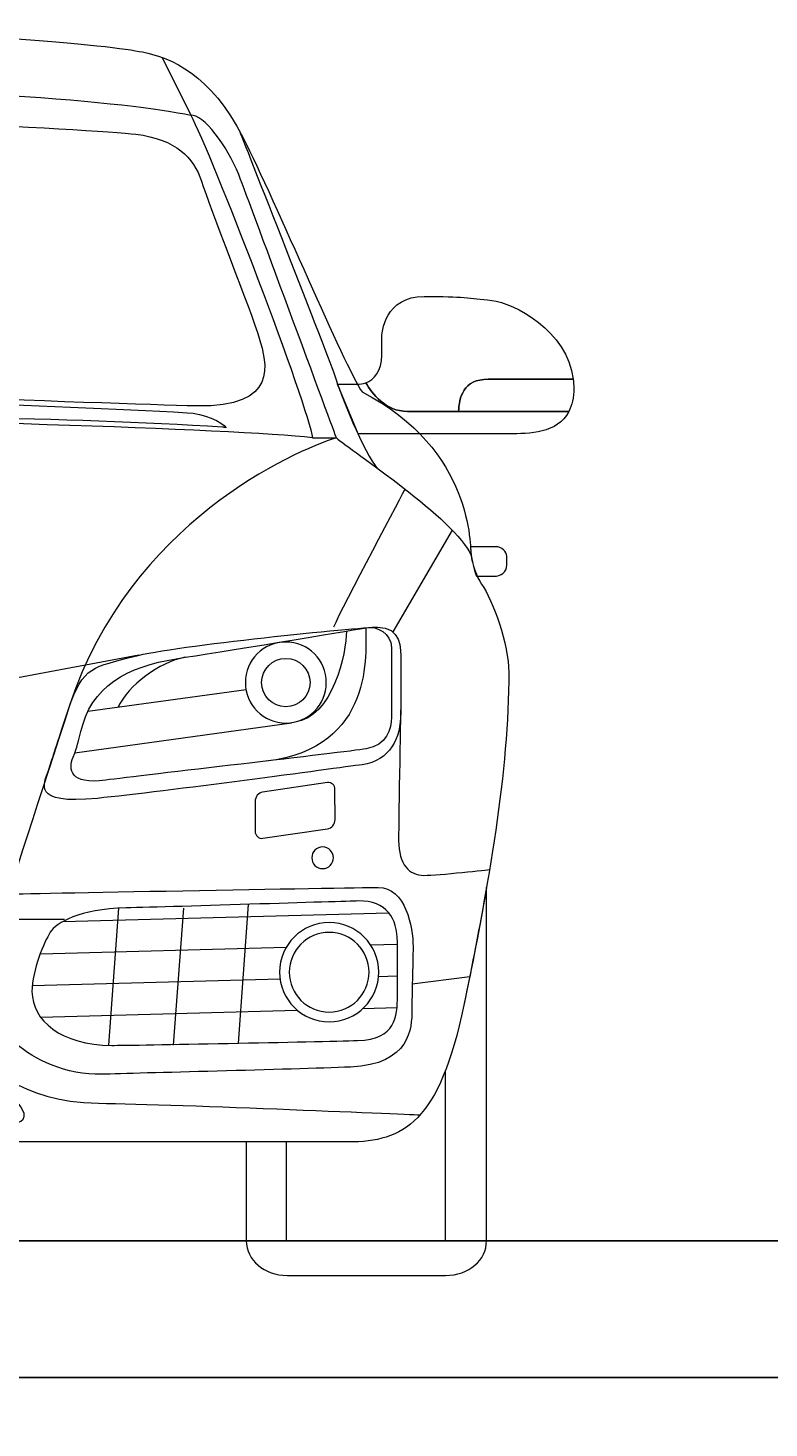
# Model space of a CAD drawing. Units: inches. Extents: x 1152 to 2588, y 1459 to 2618.
# Tile 11 of 17: x 1352 to 1384, y 2319 to 2381. Entities that reach past the tile are written whole.
import ezdxf

# ---------------------------------------------------------------- set-up
doc = ezdxf.new("R2010")
doc.units = ezdxf.units.IN
for name, color, linetype, lineweight in [('A-ANNO-DIMS', 2, 'Continuous', 18), ('A-ELEV', 7, 'Continuous', 25), ('AUDI', 7, 'Continuous', 13)]:
    doc.layers.add(name, color=color, linetype=linetype, lineweight=lineweight)
doc.styles.get("Standard").update_dxf_attribs({"font": 'arial.ttf'})
doc.dimstyles.get("Standard").update_dxf_attribs({"dimtxt": 0.18, "dimasz": 0.18, "dimexe": 0.18, "dimexo": 0.0625, "dimgap": 0.09, "dimtad": 0, "dimtih": 1, "dimtoh": 1, "dimdec": 4, "dimzin": 0, "dimdsep": 46, "dimtxsty": 'Standard', "dimcen": 0.09, "dimadec": 0, "dimazin": 0, "dimtfac": 1, "dimtdec": 4, "dimtofl": 0, "dimtmove": 0, "dimatfit": 3, "dimfxl": 1, "dimtolj": 1, "dimtzin": 0, "dimarcsym": 0})

# ---------------------------------------------------------------- blocks, each defined once
blk = doc.blocks.new('*D91')
at = {"layer": 'A-ANNO-DIMS', "color": 0, "lineweight": -2, "transparency": 16777216}
for p, q in [((1405.417, 2327.329), (1405.417, 2232.94)), ((1276.417, 2321.329), (1276.417, 2232.94)), ((1276.597, 2233.12), (1340.636, 2233.12)), ((1405.237, 2233.12), (1341.197, 2233.12))]:
    blk.add_line(p, q, dxfattribs=at)
at = {"layer": 'A-ANNO-DIMS', "color": 0, "transparency": 16777216}
for points in [[(1276.597, 2233.15), (1276.597, 2233.09), (1276.417, 2233.12)], [(1405.237, 2233.15), (1405.237, 2233.09), (1405.417, 2233.12)]]:
    blk.add_solid(points, dxfattribs=at)
at = {"layer": 'Defpoints', "color": 0, "transparency": 16777216}
for p in [(1405.417, 2327.391), (1276.417, 2321.391), (1405.417, 2233.12)]:
    blk.add_point(p, dxfattribs=at)
at = {"layer": 'A-ANNO-DIMS', "color": 0, "transparency": 16777216, "insert": (1340.917, 2233.12), "char_height": 0.18, "attachment_point": 5}
blk.add_mtext('\\A1;129', dxfattribs=at)

msp = doc.modelspace()

# ---------------------------------------------------------------- linework, layer by layer
at = {"layer": 'A-ELEV'}
for p, q in [((1736.4165, 2327.3911), (1285.4165, 2327.3911)), ((1736.4165, 2321.3911), (1276.4165, 2321.3911))]:
    msp.add_line(p, q, dxfattribs=at)
at = {"layer": 'AUDI'}
for points, knots in [([(1335.9514, 2380.6082), (1323.07, 2380.6082), (1316.2344, 2379.8209), (1314.9649, 2379.5565), (1314.9649, 2379.5565), (1313.6952, 2379.292), (1311.974, 2378.5979), (1310.5458, 2375.7943), (1310.5458, 2375.7943), (1309.1176, 2372.9909), (1306.1088, 2365.771), (1305.3217, 2364.6395), (1305.3217, 2364.6395), (1300.4024, 2362.1057), (1300.5918, 2357.8087), (1300.5428, 2357.4642), (1300.5428, 2357.4642), (1300.4936, 2357.1198), (1300.2995, 2356.5002), (1300.0824, 2356.2017), (1300.0824, 2356.2017), (1299.5785, 2355.5088), (1298.8858, 2353.5262), (1298.8858, 2352.3397), (1298.8858, 2352.3397), (1298.8858, 2347.9967), (1299.7554, 2343.0506), (1300.8566, 2337.73), (1300.8566, 2337.73), (1301.9224, 2332.5811), (1303.5104, 2331.7248), (1305.9177, 2331.7248), (1305.9177, 2331.7248), (1307.7191, 2331.725), (1335.9514, 2331.7248), (1335.9514, 2331.7248), (1335.9514, 2331.7248), (1335.9514, 2331.725), (1364.1837, 2331.7248), (1365.9852, 2331.7248), (1365.9852, 2331.7248), (1368.3925, 2331.725), (1369.9807, 2332.581), (1371.0466, 2337.73), (1371.0466, 2337.73), (1372.1483, 2343.0506), (1373.0181, 2347.9966), (1373.0181, 2352.3397), (1373.0181, 2352.3397), (1373.0181, 2353.5264), (1372.3251, 2355.5087), (1371.8212, 2356.2017), (1371.8212, 2356.2017), (1371.6039, 2356.5003), (1371.41, 2357.1198), (1371.3608, 2357.4642), (1371.3608, 2357.4642), (1371.3116, 2357.8087), (1371.501, 2362.1057), (1366.5811, 2364.6395), (1366.5811, 2364.6395), (1365.7941, 2365.7711), (1362.7853, 2372.9908), (1361.357, 2375.7943), (1361.357, 2375.7943), (1359.9288, 2378.5979), (1358.2076, 2379.292), (1356.9379, 2379.5565), (1356.9379, 2379.5565), (1355.6684, 2379.821), (1348.8329, 2380.608), (1335.9514, 2380.6082)], [0, 0, 0, 0, 0.0555556, 0.0555556, 0.0555556, 0.0555556, 0.1111111, 0.1111111, 0.1111111, 0.1111111, 0.1666667, 0.1666667, 0.1666667, 0.1666667, 0.2222222, 0.2222222, 0.2222222, 0.2222222, 0.2777778, 0.2777778, 0.2777778, 0.2777778, 0.3333333, 0.3333333, 0.3333333, 0.3333333, 0.3888889, 0.3888889, 0.3888889, 0.3888889, 0.4444444, 0.4444444, 0.4444444, 0.4444445, 0.5, 0.5, 0.5, 0.5, 0.5555556, 0.5555556, 0.5555556, 0.5555556, 0.6111111, 0.6111111, 0.6111111, 0.6111111, 0.6666667, 0.6666667, 0.6666667, 0.6666667, 0.7222222, 0.7222222, 0.7222222, 0.7222222, 0.7777778, 0.7777778, 0.7777778, 0.7777778, 0.8333333, 0.8333333, 0.8333333, 0.8333333, 0.8888889, 0.8888889, 0.8888889, 0.8888889, 0.9444444, 0.9444444, 0.9444444, 0.9444445, 1, 1, 1, 1]), ([(1335.9514, 2380.6082), (1323.07, 2380.6082), (1316.2344, 2379.8209), (1314.9649, 2379.5565), (1314.9649, 2379.5565), (1313.6952, 2379.292), (1311.974, 2378.5979), (1310.5458, 2375.7943), (1310.5458, 2375.7943), (1309.1176, 2372.9909), (1306.1088, 2365.771), (1305.3217, 2364.6395), (1305.3217, 2364.6395), (1300.4024, 2362.1057), (1300.5918, 2357.8087), (1300.5428, 2357.4642), (1300.5428, 2357.4642), (1300.4936, 2357.1198), (1300.2995, 2356.5002), (1300.0824, 2356.2017), (1300.0824, 2356.2017), (1299.5785, 2355.5088), (1298.8858, 2353.5262), (1298.8858, 2352.3397), (1298.8858, 2352.3397), (1298.8858, 2347.9967), (1299.7554, 2343.0506), (1300.8566, 2337.73), (1300.8566, 2337.73), (1301.9224, 2332.5811), (1303.5104, 2331.7248), (1305.9177, 2331.7248), (1305.9177, 2331.7248), (1307.7191, 2331.725), (1335.9514, 2331.7248), (1335.9514, 2331.7248), (1335.9514, 2331.7248), (1335.9514, 2331.7248), (1364.1837, 2331.7248), (1365.9852, 2331.7248), (1365.9852, 2331.7248), (1368.3925, 2331.725), (1369.9807, 2332.581), (1371.0466, 2337.73), (1371.0466, 2337.73), (1372.1483, 2343.0506), (1373.0181, 2347.9966), (1373.0181, 2352.3397), (1373.0181, 2352.3397), (1373.0181, 2353.5264), (1372.3251, 2355.5087), (1371.8212, 2356.2017), (1371.8212, 2356.2017), (1371.6039, 2356.5003), (1371.41, 2357.1198), (1371.3608, 2357.4642), (1371.3608, 2357.4642), (1371.3116, 2357.8087), (1371.501, 2362.1057), (1366.5811, 2364.6395), (1366.5811, 2364.6395), (1365.7941, 2365.7711), (1362.7853, 2372.9908), (1361.357, 2375.7943), (1361.357, 2375.7943), (1359.9288, 2378.5979), (1358.2076, 2379.292), (1356.9379, 2379.5565), (1356.9379, 2379.5565), (1355.6684, 2379.821), (1348.8329, 2380.608), (1335.9514, 2380.6082)], [0, 0, 0, 0, 0.0555556, 0.0555556, 0.0555556, 0.0555556, 0.1111111, 0.1111111, 0.1111111, 0.1111111, 0.1666667, 0.1666667, 0.1666667, 0.1666667, 0.2222222, 0.2222222, 0.2222222, 0.2222222, 0.2777778, 0.2777778, 0.2777778, 0.2777778, 0.3333333, 0.3333333, 0.3333333, 0.3333333, 0.3888889, 0.3888889, 0.3888889, 0.3888889, 0.4444444, 0.4444444, 0.4444444, 0.4444445, 0.5, 0.5, 0.5, 0.5, 0.5555556, 0.5555556, 0.5555556, 0.5555556, 0.6111111, 0.6111111, 0.6111111, 0.6111111, 0.6666667, 0.6666667, 0.6666667, 0.6666667, 0.7222222, 0.7222222, 0.7222222, 0.7222222, 0.7777778, 0.7777778, 0.7777778, 0.7777778, 0.8333333, 0.8333333, 0.8333333, 0.8333333, 0.8888889, 0.8888889, 0.8888889, 0.8888889, 0.9444444, 0.9444444, 0.9444444, 0.9444445, 1, 1, 1, 1]), ([(1335.9514, 2378.0831), (1323.862, 2378.0831), (1315.9013, 2377.3042), (1312.8453, 2376.7794), (1312.8453, 2376.7794), (1311.9763, 2375.2275), (1307.631, 2363.8673), (1307.5068, 2362.6256), (1307.5068, 2362.6256), (1310.8591, 2362.9982), (1325.7217, 2363.4947), (1335.9514, 2363.4947), (1335.9514, 2363.4947), (1346.1812, 2363.4947), (1361.0438, 2362.998), (1364.396, 2362.6256), (1364.396, 2362.6256), (1364.2719, 2363.8675), (1359.9266, 2375.2274), (1359.0575, 2376.7794), (1359.0575, 2376.7794), (1356.4376, 2377.3639), (1348.0408, 2378.0829), (1335.9514, 2378.0831)], [0, 0, 0, 0, 0.1666667, 0.1666667, 0.1666667, 0.1666667, 0.3333333, 0.3333333, 0.3333333, 0.3333333, 0.5, 0.5, 0.5, 0.5, 0.6666667, 0.6666667, 0.6666667, 0.6666667, 0.8333333, 0.8333333, 0.8333333, 0.8333333, 1, 1, 1, 1]), ([(1335.9514, 2376.8669), (1331.6617, 2376.8669), (1317.0146, 2376.1677), (1315.2481, 2375.9467), (1315.2481, 2375.9467), (1313.4816, 2375.7259), (1312.7088, 2374.9163), (1312.3775, 2373.8859), (1312.3775, 2373.8859), (1312.0463, 2372.8554), (1310.1695, 2368.1078), (1309.8383, 2367.0037), (1309.8383, 2367.0037), (1309.5071, 2365.8998), (1308.9561, 2363.9401), (1312.5985, 2364.0229), (1312.5985, 2364.0229), (1316.4298, 2364.1101), (1333.6902, 2364.7958), (1335.9514, 2364.7958), (1335.9514, 2364.7958), (1338.2126, 2364.7959), (1355.473, 2364.1101), (1359.3043, 2364.0229), (1359.3043, 2364.0229), (1362.9467, 2363.9401), (1362.3958, 2365.8997), (1362.0646, 2367.0037), (1362.0646, 2367.0037), (1361.7334, 2368.1079), (1359.8565, 2372.8554), (1359.5253, 2373.8859), (1359.5253, 2373.8859), (1359.1941, 2374.9164), (1358.4212, 2375.7259), (1356.6547, 2375.9467), (1356.6547, 2375.9467), (1354.8882, 2376.1677), (1340.2411, 2376.8668), (1335.9514, 2376.8669)], [0, 0, 0, 0, 0.1, 0.1, 0.1, 0.1, 0.2, 0.2, 0.2, 0.2, 0.3, 0.3, 0.3, 0.3, 0.4, 0.4, 0.4, 0.4, 0.5, 0.5, 0.5, 0.5, 0.6, 0.6, 0.6, 0.6, 0.7, 0.7, 0.7, 0.7, 0.8, 0.8, 0.8, 0.8, 0.9, 0.9, 0.9, 0.9, 1, 1, 1, 1]), ([(1364.396, 2362.6256), (1364.2719, 2363.8675), (1359.9266, 2375.2274), (1359.0575, 2376.7794), (1359.0575, 2376.7794), (1359.616, 2376.8414), (1360.6567, 2375.4309), (1361.168, 2374.1721), (1361.168, 2374.1721), (1361.3562, 2373.7086), (1365.4512, 2362.6256), (1365.4512, 2362.6256), (1365.4512, 2362.6256), (1365.4512, 2362.6256), (1364.396, 2362.6256), (1364.396, 2362.6256)], [0, 0, 0, 0, 0.25, 0.25, 0.25, 0.25, 0.5, 0.5, 0.5, 0.5, 0.75, 0.75, 0.75, 0.75, 1, 1, 1, 1]), ([(1361.2043, 2376.0821), (1361.2043, 2376.0821), (1365.2184, 2365.9026), (1365.3948, 2365.3031), (1365.3948, 2365.3031), (1365.5714, 2364.7035), (1366.6742, 2361.8719), (1367.2738, 2361.2722)], [0, 0, 0, 0, 0.5, 0.5, 0.5, 0.5, 1, 1, 1, 1]), ([(1372.1131, 2365.1973), (1373.0816, 2365.1973), (1374.868, 2365.1973), (1375.8424, 2365.1973), (1375.8424, 2365.1973), (1375.5815, 2367.3215), (1373.237, 2368.5533), (1372.2716, 2368.6531), (1372.2716, 2368.6531), (1371.2487, 2368.759), (1371.0374, 2368.8293), (1369.3093, 2368.8293), (1369.3093, 2368.8293), (1367.5813, 2368.8294), (1367.4403, 2367.2778), (1367.4403, 2366.925), (1367.4403, 2366.925), (1367.4403, 2366.5723), (1367.4403, 2366.7135), (1367.4403, 2366.2552), (1367.4403, 2366.2552), (1367.4403, 2365.5383), (1367.1204, 2365.1733), (1366.7397, 2365.0364), (1366.7397, 2365.0364), (1367.0228, 2364.5611), (1367.5973, 2363.7821), (1368.5737, 2363.7821), (1368.5737, 2363.7821), (1368.9566, 2363.7822), (1369.8088, 2363.7821), (1370.8123, 2363.7821), (1370.8123, 2363.7821), (1370.8382, 2364.3736), (1371.0125, 2365.1973), (1372.1131, 2365.1973)], [0, 0, 0, 0, 0.1111111, 0.1111111, 0.1111111, 0.1111111, 0.2222222, 0.2222222, 0.2222222, 0.2222222, 0.3333333, 0.3333333, 0.3333333, 0.3333333, 0.4444444, 0.4444444, 0.4444444, 0.4444445, 0.5555556, 0.5555556, 0.5555556, 0.5555556, 0.6666667, 0.6666667, 0.6666667, 0.6666667, 0.7777778, 0.7777778, 0.7777778, 0.7777778, 0.8888889, 0.8888889, 0.8888889, 0.8888889, 1, 1, 1, 1]), ([(1368.5737, 2363.7822), (1367.5973, 2363.7822), (1367.0228, 2364.561), (1366.7397, 2365.0364), (1366.7397, 2365.0364), (1366.6147, 2364.9918), (1366.4834, 2364.9709), (1366.3545, 2364.9709), (1366.3545, 2364.9709), (1365.833, 2364.971), (1365.5006, 2364.9709), (1365.5006, 2364.9709), (1365.5006, 2364.9709), (1365.5006, 2364.9709), (1366.4076, 2362.7992), (1366.4076, 2362.7992), (1366.4076, 2362.7992), (1366.4076, 2362.7992), (1371.8837, 2362.7991), (1373.0181, 2362.7991), (1373.0181, 2362.7991), (1373.9106, 2362.7992), (1375.1595, 2362.8035), (1375.6533, 2363.7821), (1375.6533, 2363.7821), (1373.9943, 2363.7822), (1369.6003, 2363.7821), (1368.5737, 2363.7822)], [0, 0, 0, 0, 0.1428571, 0.1428571, 0.1428571, 0.1428572, 0.2857143, 0.2857143, 0.2857143, 0.2857143, 0.4285714, 0.4285714, 0.4285714, 0.4285714, 0.5714286, 0.5714286, 0.5714286, 0.5714286, 0.7142857, 0.7142857, 0.7142857, 0.7142857, 0.8571429, 0.8571429, 0.8571429, 0.8571429, 1, 1, 1, 1]), ([(1372.1131, 2365.1973), (1371.0127, 2365.1973), (1370.8381, 2364.3735), (1370.8123, 2363.7821), (1370.8123, 2363.7821), (1372.4987, 2363.7822), (1374.6133, 2363.7821), (1375.6533, 2363.7821), (1375.6533, 2363.7821), (1375.7871, 2364.0477), (1375.8686, 2364.3803), (1375.8686, 2364.8092), (1375.8686, 2364.8092), (1375.8686, 2364.9422), (1375.8578, 2365.0706), (1375.8424, 2365.1973), (1375.8424, 2365.1973), (1374.868, 2365.1973), (1373.0816, 2365.1973), (1372.1131, 2365.1973)], [0, 0, 0, 0, 0.2, 0.2, 0.2, 0.2, 0.4, 0.4, 0.4, 0.4, 0.6, 0.6, 0.6, 0.6, 0.8, 0.8, 0.8, 0.8, 1, 1, 1, 1]), ([(1360.6101, 2363.0565), (1360.4577, 2363.3307), (1359.6046, 2363.696), (1358.9039, 2363.7266), (1358.9039, 2363.7266), (1352.6576, 2364.0622), (1343.4864, 2364.4578), (1338.4895, 2363.9399), (1338.4895, 2363.9399), (1338.2456, 2363.9094), (1338.063, 2363.7572), (1338.0934, 2363.6353), (1338.0934, 2363.6353), (1345.3146, 2363.5742), (1353.4498, 2363.5438), (1360.4577, 2363.0868), (1360.4577, 2363.0868), (1360.5188, 2363.087), (1360.5491, 2363.0868), (1360.6101, 2363.0565)], [0, 0, 0, 0, 0.2, 0.2, 0.2, 0.2, 0.4, 0.4, 0.4, 0.4, 0.6, 0.6, 0.6, 0.6, 0.8, 0.8, 0.8, 0.8, 1, 1, 1, 1]), ([(1360.6101, 2363.0565), (1360.4577, 2363.3307), (1359.6046, 2363.696), (1358.9039, 2363.7266), (1358.9039, 2363.7266), (1352.6576, 2364.0622), (1343.4864, 2364.4578), (1338.4895, 2363.9399), (1338.4895, 2363.9399), (1338.2456, 2363.9094), (1338.063, 2363.7572), (1338.0934, 2363.6353), (1338.0934, 2363.6353), (1345.3146, 2363.5742), (1353.4498, 2363.5438), (1360.4577, 2363.0868), (1360.4577, 2363.0868), (1360.5188, 2363.087), (1360.5491, 2363.0868), (1360.6101, 2363.0565)], [0, 0, 0, 0, 0.2, 0.2, 0.2, 0.2, 0.4, 0.4, 0.4, 0.4, 0.6, 0.6, 0.6, 0.6, 0.8, 0.8, 0.8, 0.8, 1, 1, 1, 1]), ([(1360.6101, 2363.0565), (1360.4577, 2363.3307), (1359.6046, 2363.696), (1358.9039, 2363.7266), (1358.9039, 2363.7266), (1352.6576, 2364.0622), (1343.4864, 2364.4578), (1338.4895, 2363.9399), (1338.4895, 2363.9399), (1338.2456, 2363.9094), (1338.063, 2363.7572), (1338.0934, 2363.6353), (1338.0934, 2363.6353), (1345.3146, 2363.5742), (1353.4498, 2363.5438), (1360.4577, 2363.0868), (1360.4577, 2363.0868), (1360.5188, 2363.087), (1360.5491, 2363.0868), (1360.6101, 2363.0565)], [0, 0, 0, 0, 0.2, 0.2, 0.2, 0.2, 0.4, 0.4, 0.4, 0.4, 0.6, 0.6, 0.6, 0.6, 0.8, 0.8, 0.8, 0.8, 1, 1, 1, 1]), ([(1365.4513, 2362.6256), (1363.6317, 2362.0587), (1356.3668, 2358.8847), (1353.7573, 2350.9148), (1353.7573, 2350.9148), (1351.1478, 2342.9449), (1348.8633, 2335.7722), (1348.8633, 2335.7722)], [0, 0, 0, 0, 0.5, 0.5, 0.5, 0.5, 1, 1, 1, 1]), ([(1371.3381, 2357.8463), (1371.3381, 2357.8463), (1372.1189, 2357.8463), (1372.4232, 2357.8463), (1372.4232, 2357.8463), (1372.7276, 2357.8463), (1372.9262, 2357.6221), (1372.9262, 2357.4235), (1372.9262, 2357.4235), (1372.9262, 2357.225), (1372.9262, 2357.4132), (1372.9262, 2357.0433), (1372.9262, 2357.0433), (1372.9262, 2356.708), (1372.6769, 2356.5507), (1372.3592, 2356.5507), (1372.3592, 2356.5507), (1372.0414, 2356.5508), (1371.6033, 2356.5562), (1371.6033, 2356.5562), (1371.6033, 2356.5562), (1371.6033, 2356.5564), (1371.3385, 2357.2497), (1371.3381, 2357.8463)], [0, 0, 0, 0, 0.1666667, 0.1666667, 0.1666667, 0.1666667, 0.3333333, 0.3333333, 0.3333333, 0.3333333, 0.5, 0.5, 0.5, 0.5, 0.6666667, 0.6666667, 0.6666667, 0.6666667, 0.8333333, 0.8333333, 0.8333333, 0.8333333, 1, 1, 1, 1]), ([(1371.3381, 2357.8463), (1371.3381, 2357.8463), (1372.1189, 2357.8463), (1372.4232, 2357.8463), (1372.4232, 2357.8463), (1372.7276, 2357.8463), (1372.9262, 2357.6221), (1372.9262, 2357.4235), (1372.9262, 2357.4235), (1372.9262, 2357.225), (1372.9262, 2357.4132), (1372.9262, 2357.0433), (1372.9262, 2357.0433), (1372.9262, 2356.708), (1372.6769, 2356.5507), (1372.3592, 2356.5507), (1372.3592, 2356.5507), (1372.0414, 2356.5508), (1371.6033, 2356.5562), (1371.6033, 2356.5562), (1371.6033, 2356.5562), (1371.6033, 2356.5562), (1371.3381, 2357.2497), (1371.3381, 2357.8463)], [0, 0, 0, 0, 0.1666667, 0.1666667, 0.1666667, 0.1666667, 0.3333333, 0.3333333, 0.3333333, 0.3333333, 0.5, 0.5, 0.5, 0.5, 0.6666667, 0.6666667, 0.6666667, 0.6666667, 0.8333333, 0.8333333, 0.8333333, 0.8333333, 1, 1, 1, 1]), ([(1367.2498, 2354.3162), (1366.4995, 2354.3162), (1358.302, 2353.5024), (1356.5681, 2353.0315), (1356.5681, 2353.0315), (1354.8344, 2352.5608), (1354.3206, 2352.6395), (1353.69, 2350.7088), (1353.69, 2350.7088), (1353.0594, 2348.7781), (1352.9899, 2348.5655), (1352.812, 2348.0188), (1352.812, 2348.0188), (1352.6341, 2347.4722), (1352.0088, 2346.5027), (1354.9628, 2346.8024), (1354.9628, 2346.8024), (1357.9169, 2347.102), (1365.3661, 2348.1084), (1366.5862, 2348.2794), (1366.5862, 2348.2794), (1367.8064, 2348.4506), (1368.2774, 2349.4353), (1368.2774, 2350.5484), (1368.2774, 2350.5484), (1368.2774, 2351.6615), (1368.2774, 2352.175), (1368.2774, 2352.7959), (1368.2774, 2352.7959), (1368.2774, 2353.4171), (1368.2984, 2354.3159), (1367.2498, 2354.3162)], [0, 0, 0, 0, 0.125, 0.125, 0.125, 0.125, 0.25, 0.25, 0.25, 0.25, 0.375, 0.375, 0.375, 0.375, 0.5, 0.5, 0.5, 0.5, 0.625, 0.625, 0.625, 0.625, 0.75, 0.75, 0.75, 0.75, 0.875, 0.875, 0.875, 0.875, 1, 1, 1, 1]), ([(1366.7393, 2354.2871), (1366.7393, 2354.2871), (1360.9867, 2353.3127), (1358.8179, 2352.9953), (1358.8179, 2352.9953), (1356.6491, 2352.6781), (1354.9035, 2351.9903), (1354.3217, 2350.0331), (1354.3217, 2350.0331), (1354.0572, 2349.134), (1354.1101, 2349.1338), (1353.8985, 2348.6049), (1353.8985, 2348.6049), (1353.6869, 2348.0759), (1353.7398, 2347.3881), (1355.3267, 2347.5998), (1355.3267, 2347.5998), (1356.9137, 2347.8115), (1365.8035, 2348.8166), (1366.7526, 2348.9752), (1366.7526, 2348.9752), (1367.6789, 2349.1299), (1367.8635, 2349.8403), (1367.8635, 2350.3693), (1367.8635, 2350.3693), (1367.8635, 2350.8983), (1367.8635, 2352.7796), (1367.8635, 2353.4185), (1367.8635, 2353.4185), (1367.8635, 2354.0577), (1367.2527, 2354.3736), (1366.7393, 2354.2871)], [0, 0, 0, 0, 0.125, 0.125, 0.125, 0.125, 0.25, 0.25, 0.25, 0.25, 0.375, 0.375, 0.375, 0.375, 0.5, 0.5, 0.5, 0.5, 0.625, 0.625, 0.625, 0.625, 0.75, 0.75, 0.75, 0.75, 0.875, 0.875, 0.875, 0.875, 1, 1, 1, 1]), ([(1361.4567, 2351.8838), (1361.4567, 2352.8648), (1362.2518, 2353.6599), (1363.2328, 2353.6599), (1363.2328, 2353.6599), (1364.214, 2353.6601), (1365.0093, 2352.8648), (1365.0093, 2351.8837), (1365.0093, 2351.8837), (1365.0093, 2350.9027), (1364.214, 2350.1072), (1363.2328, 2350.1072), (1363.2328, 2350.1072), (1362.2518, 2350.1073), (1361.4567, 2350.9025), (1361.4567, 2351.8838)], [0, 0, 0, 0, 0.25, 0.25, 0.25, 0.25, 0.5, 0.5, 0.5, 0.5, 0.75, 0.75, 0.75, 0.75, 1, 1, 1, 1]), ([(1364.2956, 2351.8838), (1364.2956, 2352.4706), (1363.8199, 2352.9461), (1363.2328, 2352.9461), (1363.2328, 2352.9461), (1362.646, 2352.9463), (1362.1704, 2352.4705), (1362.1704, 2351.8837), (1362.1704, 2351.8837), (1362.1704, 2351.2966), (1362.646, 2350.821), (1363.2328, 2350.821), (1363.2328, 2350.821), (1363.8199, 2350.821), (1364.2956, 2351.2966), (1364.2956, 2351.8838)], [0, 0, 0, 0, 0.25, 0.25, 0.25, 0.25, 0.5, 0.5, 0.5, 0.5, 0.75, 0.75, 0.75, 0.75, 1, 1, 1, 1]), ([(1368.2774, 2351.0383), (1368.2774, 2351.0383), (1368.1808, 2346.0128), (1368.1808, 2344.9549), (1368.1808, 2344.9549), (1368.1808, 2343.8971), (1368.6569, 2343.4208), (1369.2917, 2343.4208), (1369.2917, 2343.4208), (1369.9266, 2343.421), (1372.1767, 2343.6806), (1372.1767, 2343.6806)], [0, 0, 0, 0, 0.3333333, 0.3333333, 0.3333333, 0.3333333, 0.6666667, 0.6666667, 0.6666667, 0.6666667, 1, 1, 1, 1]), ([(1365.3912, 2345.8748), (1365.3912, 2345.6736), (1365.2432, 2345.489), (1365.0604, 2345.4624), (1365.0604, 2345.4624), (1365.0604, 2345.4624), (1362.2179, 2345.048), (1362.2179, 2345.048), (1362.2179, 2345.048), (1362.035, 2345.0214), (1361.8864, 2345.1626), (1361.8864, 2345.3636), (1361.8864, 2345.3636), (1361.8864, 2345.3636), (1361.8852, 2346.6682), (1361.8852, 2346.6682), (1361.8852, 2346.6682), (1361.8852, 2346.8693), (1362.0334, 2347.0536), (1362.2162, 2347.0803), (1362.2162, 2347.0803), (1362.2162, 2347.0803), (1365.0587, 2347.4949), (1365.0587, 2347.4949), (1365.0587, 2347.4949), (1365.2415, 2347.5215), (1365.3901, 2347.3801), (1365.3901, 2347.1791), (1365.3901, 2347.1791), (1365.3901, 2347.1791), (1365.3912, 2345.8748), (1365.3912, 2345.8748)], [0, 0, 0, 0, 0.125, 0.125, 0.125, 0.125, 0.25, 0.25, 0.25, 0.25, 0.375, 0.375, 0.375, 0.375, 0.5, 0.5, 0.5, 0.5, 0.625, 0.625, 0.625, 0.625, 0.75, 0.75, 0.75, 0.75, 0.875, 0.875, 0.875, 0.875, 1, 1, 1, 1]), ([(1364.3722, 2344.1942), (1364.3722, 2344.457), (1364.5855, 2344.6702), (1364.8483, 2344.6702), (1364.8483, 2344.6702), (1365.1111, 2344.6703), (1365.3244, 2344.4569), (1365.3244, 2344.194), (1365.3244, 2344.194), (1365.3244, 2343.9313), (1365.1111, 2343.7179), (1364.8483, 2343.7179), (1364.8483, 2343.7179), (1364.5855, 2343.7181), (1364.3722, 2343.9312), (1364.3722, 2344.1942)], [0, 0, 0, 0, 0.25, 0.25, 0.25, 0.25, 0.5, 0.5, 0.5, 0.5, 0.75, 0.75, 0.75, 0.75, 1, 1, 1, 1]), ([(1351.057, 2342.6054), (1351.057, 2342.6054), (1366.0649, 2342.8919), (1367.2816, 2342.8919), (1367.2816, 2342.8919), (1368.4983, 2342.8919), (1368.8156, 2341.1463), (1368.8156, 2340.2999), (1368.8156, 2340.2999), (1368.8156, 2339.4536), (1368.7627, 2338.2368), (1368.7627, 2337.4963), (1368.7627, 2337.4963), (1368.7627, 2336.7559), (1368.7098, 2335.1159), (1366.0649, 2335.0101), (1366.0649, 2335.0101), (1363.4201, 2334.9044), (1356.7549, 2334.7456), (1355.168, 2334.6927), (1355.168, 2334.6927), (1353.5811, 2334.6399), (1352.1528, 2335.3804), (1351.4122, 2336.0151), (1351.4122, 2336.0151), (1350.6717, 2336.6499), (1349.5651, 2337.9711), (1350.0415, 2339.452)], [0, 0, 0, 0, 0.1428571, 0.1428571, 0.1428571, 0.1428572, 0.2857143, 0.2857143, 0.2857143, 0.2857143, 0.4285714, 0.4285714, 0.4285714, 0.4285714, 0.5714286, 0.5714286, 0.5714286, 0.5714286, 0.7142857, 0.7142857, 0.7142857, 0.7142857, 0.8571429, 0.8571429, 0.8571429, 0.8571429, 1, 1, 1, 1]), ([(1371.0467, 2337.73), (1371.4128, 2339.4986), (1371.7488, 2341.221), (1372.0403, 2342.8986), (1372.0403, 2342.8986), (1372.0403, 2342.8986), (1372.0403, 2327.3911), (1372.0403, 2327.3911), (1372.0403, 2327.3911), (1372.0403, 2326.5378), (1371.2605, 2325.8678), (1370.2438, 2325.8678), (1370.2438, 2325.8678), (1370.2438, 2325.8678), (1363.2948, 2325.8679), (1363.2948, 2325.8679), (1363.2948, 2325.8679), (1362.2782, 2325.8679), (1361.4984, 2326.5378), (1361.4984, 2327.3909), (1361.4984, 2327.3909), (1361.4984, 2327.3909), (1361.4985, 2331.725), (1361.4985, 2331.725), (1361.4985, 2331.725), (1363.8926, 2331.725), (1365.5866, 2331.7248), (1365.9852, 2331.7248), (1365.9852, 2331.7248), (1368.3925, 2331.725), (1369.9807, 2332.581), (1371.0467, 2337.73)], [0, 0, 0, 0, 0.125, 0.125, 0.125, 0.125, 0.25, 0.25, 0.25, 0.25, 0.375, 0.375, 0.375, 0.375, 0.5, 0.5, 0.5, 0.5, 0.625, 0.625, 0.625, 0.625, 0.75, 0.75, 0.75, 0.75, 0.875, 0.875, 0.875, 0.875, 1, 1, 1, 1]), ([(1366.4105, 2342.2994), (1367.6619, 2342.3251), (1368.1279, 2341.5165), (1368.1279, 2340.5115), (1368.1279, 2340.5115), (1368.1279, 2339.5065), (1368.1279, 2339.0304), (1368.1279, 2338.131), (1368.1279, 2338.131), (1368.1279, 2337.232), (1368.075, 2336.2267), (1366.3823, 2336.1738), (1366.3823, 2336.1738), (1364.6897, 2336.121), (1356.5433, 2335.9622), (1355.5912, 2335.9622), (1355.5912, 2335.9622), (1353.3705, 2335.9623), (1352.0939, 2337.0692), (1352.0939, 2338.3206), (1352.0939, 2338.3206), (1352.0939, 2339.2729), (1352.6304, 2340.5003), (1352.8948, 2340.9235), (1352.8948, 2340.9235), (1353.1593, 2341.3467), (1354.163, 2341.9397), (1356.226, 2341.9926), (1356.226, 2341.9926), (1358.289, 2342.0456), (1366.4105, 2342.2992), (1366.4105, 2342.2994)], [0, 0, 0, 0, 0.125, 0.125, 0.125, 0.125, 0.25, 0.25, 0.25, 0.25, 0.375, 0.375, 0.375, 0.375, 0.5, 0.5, 0.5, 0.5, 0.625, 0.625, 0.625, 0.625, 0.75, 0.75, 0.75, 0.75, 0.875, 0.875, 0.875, 0.875, 1, 1, 1, 1]), ([(1366.4105, 2342.2994), (1367.6619, 2342.3251), (1368.1279, 2341.5165), (1368.1279, 2340.5115), (1368.1279, 2340.5115), (1368.1279, 2339.5065), (1368.1279, 2339.0304), (1368.1279, 2338.131), (1368.1279, 2338.131), (1368.1279, 2337.232), (1368.075, 2336.2267), (1366.3823, 2336.1738), (1366.3823, 2336.1738), (1364.6897, 2336.121), (1356.5433, 2335.9622), (1355.5912, 2335.9622), (1355.5912, 2335.9622), (1353.3705, 2335.9623), (1352.0939, 2337.0692), (1352.0939, 2338.3206), (1352.0939, 2338.3206), (1352.0939, 2339.2729), (1352.6304, 2340.5003), (1352.8948, 2340.9235), (1352.8948, 2340.9235), (1353.1593, 2341.3467), (1354.163, 2341.9397), (1356.226, 2341.9926), (1356.226, 2341.9926), (1358.289, 2342.0456), (1366.4105, 2342.2994), (1366.4105, 2342.2994)], [0, 0, 0, 0, 0.125, 0.125, 0.125, 0.125, 0.25, 0.25, 0.25, 0.25, 0.375, 0.375, 0.375, 0.375, 0.5, 0.5, 0.5, 0.5, 0.625, 0.625, 0.625, 0.625, 0.75, 0.75, 0.75, 0.75, 0.875, 0.875, 0.875, 0.875, 1, 1, 1, 1]), ([(1362.9564, 2339.1716), (1362.9564, 2340.3741), (1363.9312, 2341.3489), (1365.1339, 2341.3489), (1365.1339, 2341.3489), (1366.3365, 2341.3491), (1367.3114, 2340.374), (1367.3114, 2339.1714), (1367.3114, 2339.1714), (1367.3114, 2337.969), (1366.3365, 2336.994), (1365.1339, 2336.994), (1365.1339, 2336.994), (1363.9313, 2336.9942), (1362.9564, 2337.9689), (1362.9564, 2339.1716)], [0, 0, 0, 0, 0.25, 0.25, 0.25, 0.25, 0.5, 0.5, 0.5, 0.5, 0.75, 0.75, 0.75, 0.75, 1, 1, 1, 1]), ([(1363.3835, 2339.1716), (1363.3835, 2340.1384), (1364.1673, 2340.9218), (1365.1339, 2340.9218), (1365.1339, 2340.9218), (1366.1005, 2340.9218), (1366.8842, 2340.1383), (1366.8842, 2339.1714), (1366.8842, 2339.1714), (1366.8842, 2338.2046), (1366.1005, 2337.4211), (1365.1339, 2337.4211), (1365.1339, 2337.4211), (1364.1673, 2337.4213), (1363.3835, 2338.2046), (1363.3835, 2339.1716)], [0, 0, 0, 0, 0.25, 0.25, 0.25, 0.25, 0.5, 0.5, 0.5, 0.5, 0.75, 0.75, 0.75, 0.75, 1, 1, 1, 1]), ([(1335.9514, 2332.5064), (1335.9514, 2332.5064), (1323.0118, 2332.5064), (1321.0371, 2332.5064), (1321.0371, 2332.5064), (1319.0624, 2332.5064), (1320.896, 2333.8463), (1321.4603, 2334.5515), (1321.4603, 2334.5515), (1322.0246, 2335.257), (1323.0693, 2336.2444), (1325.6922, 2336.2444), (1325.6922, 2336.2444), (1328.3149, 2336.2444), (1335.9514, 2336.2444), (1335.9514, 2336.2444), (1335.9514, 2336.2444), (1335.9514, 2336.2444), (1343.5879, 2336.2444), (1346.2106, 2336.2444), (1346.2106, 2336.2444), (1348.8335, 2336.2444), (1349.8782, 2335.2569), (1350.4425, 2334.5515), (1350.4425, 2334.5515), (1351.0069, 2333.8463), (1352.8404, 2332.5064), (1350.8657, 2332.5064), (1350.8657, 2332.5064), (1348.891, 2332.5064), (1335.9514, 2332.5064), (1335.9514, 2332.5064)], [0, 0, 0, 0, 0.125, 0.125, 0.125, 0.125, 0.25, 0.25, 0.25, 0.25, 0.375, 0.375, 0.375, 0.375, 0.5, 0.5, 0.5, 0.5, 0.625, 0.625, 0.625, 0.625, 0.75, 0.75, 0.75, 0.75, 0.875, 0.875, 0.875, 0.875, 1, 1, 1, 1]), ([(1349.1541, 2335.6318), (1350.3014, 2335.2217), (1351.4122, 2333.4761), (1355.0093, 2333.4232), (1355.0093, 2333.4232), (1358.6063, 2333.3703), (1369.1239, 2332.9116), (1369.1239, 2332.9116)], [0, 0, 0, 0, 0.5, 0.5, 0.5, 0.5, 1, 1, 1, 1])]:
    msp.add_open_spline(points, degree=3, knots=knots, dxfattribs=at)
for points in [[(1357.8115, 2379.308), (1357.8115, 2379.308), (1359.0575, 2376.7795), (1359.0575, 2376.7795)], [(1365.4513, 2362.6256), (1366.0296, 2362.0938), (1370.6964, 2359.058), (1371.3608, 2357.4642)], [(1368.4644, 2360.3723), (1368.4644, 2360.3723), (1365.6947, 2355.1641), (1365.3244, 2354.3178)], [(1370.5337, 2358.5742), (1370.5337, 2358.5742), (1367.9214, 2354.1126), (1367.9214, 2354.1126)], [(1366.7393, 2354.2871), (1366.7393, 2353.2599), (1367.1578, 2348.9973), (1362.3757, 2348.4362)], [(1365.891, 2354.1443), (1365.891, 2353.2072), (1365.2934, 2350.3368), (1363.6234, 2350.1515)], [(1356.7845, 2353.0848), (1356.7845, 2353.0848), (1351.2418, 2352.0479), (1351.2418, 2352.0479)], [(1358.818, 2352.9954), (1357.6614, 2352.7751), (1356.3371, 2351.7638), (1355.8583, 2350.7927)], [(1361.4865, 2351.5677), (1361.4865, 2351.5677), (1354.5484, 2350.6122), (1354.5484, 2350.6122)], [(1363.4839, 2350.1073), (1363.4839, 2350.1073), (1353.9691, 2348.7882), (1353.9691, 2348.7882)], [(1361.5864, 2342.1503), (1361.5864, 2342.1503), (1361.1417, 2336.0567), (1361.1417, 2336.0567)], [(1353.5184, 2341.4908), (1353.5184, 2341.4908), (1350.7172, 2341.4908), (1350.7172, 2341.4908)], [(1353.4534, 2341.397), (1353.4534, 2341.397), (1367.7501, 2341.7769), (1367.7501, 2341.7769)], [(1355.8956, 2341.979), (1355.8956, 2341.979), (1355.4465, 2335.9649), (1355.4465, 2335.9649)], [(1358.7398, 2341.979), (1358.7398, 2341.979), (1358.2908, 2335.9649), (1358.2908, 2335.9649)], [(1352.468, 2339.9823), (1352.468, 2339.9823), (1363.2539, 2340.2694), (1363.2539, 2340.2694)], [(1366.9531, 2340.3676), (1366.9531, 2340.3676), (1368.1118, 2340.3984), (1368.1118, 2340.3984)], [(1367.3036, 2338.989), (1367.3036, 2338.989), (1368.1118, 2339.0098), (1368.1118, 2339.0098)], [(1368.7841, 2338.6623), (1368.7841, 2338.6623), (1371.3016, 2338.9776), (1371.3016, 2338.9776)], [(1352.1065, 2338.5941), (1352.1065, 2338.5941), (1362.9773, 2338.8766), (1362.9773, 2338.8766)], [(1352.468, 2337.2056), (1352.468, 2337.2056), (1363.7327, 2337.505), (1363.7327, 2337.505)], [(1366.6193, 2337.5819), (1366.6193, 2337.5819), (1368.1118, 2337.6217), (1368.1118, 2337.6217)], [(1370.244, 2327.3911), (1370.244, 2327.3911), (1370.244, 2334.8073), (1370.244, 2334.8073)], [(1363.2611, 2327.3911), (1363.2611, 2327.3911), (1363.2611, 2331.725), (1363.2611, 2331.725)]]:
    msp.add_open_spline(points, degree=3, dxfattribs=at)

# ---------------------------------------------------------------- dimensions: what is measured, and where the dimension line sits
at = {"layer": 'A-ANNO-DIMS'}
dim = msp.add_linear_dim(base=(1405.4165, 2233.12), p1=(1276.4165, 2321.3911), p2=(1405.4165, 2327.3911), dimstyle='Standard', override={"dimdec": 0, "dimlfac": 1, "dimrnd": 0, "dimzin": 0, "dimdsep": 46, "dimlunit": 2}, dxfattribs=at)
dim.commit()
dim.dimension.update_dxf_attribs({"geometry": '*D91', "text_midpoint": (1340.9165, 2233.12)})

doc.saveas('drawing.dxf')
